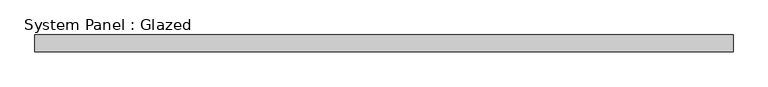
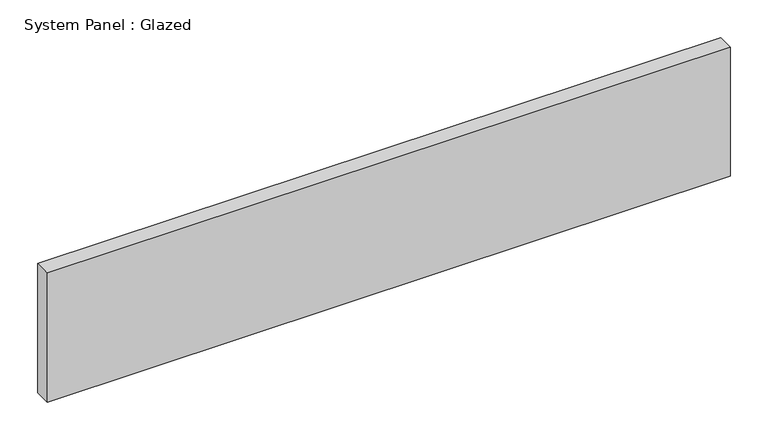
"""IFC4 building model written with IfcOpenShell, lengths in millimetres: plate geometry, System Panel : Glazed."""

from ifc_helpers import new_model, si_unit, origin, origin_with_axes, place, context, project, spatial, polyline, outline, extrude, source, transform, mapped, element, save


def system_panel_glazed_6ba3ac31(model_context):
    return source(origin(), model_context, "Body", "SweptSolid", [
        extrude(outline(polyline([(523.875, 19.05), (-523.875, 19.05), (-523.875, 44.45), (523.875, 44.45), (523.875, 19.05)])), origin_with_axes(), (0.0, 0.0, 1.0), 209.55),
    ])


if __name__ == "__main__":
    model = new_model("IFC4")
    model_context = context("Model", 3, world=origin())
    ifc_project = project(units=[si_unit("LENGTHUNIT", "METRE", prefix="MILLI")], contexts=[model_context])
    site = spatial("IfcSite", under=ifc_project)
    building = spatial("IfcBuilding", under=site)
    placement = place(None, origin())
    system_panel_glazed_shape = system_panel_glazed_6ba3ac31(model_context)
    element("IfcPlate", 1, ObjectType="System Panel : Glazed", at=placement, inside=building, context=model_context, shape_type="MappedRepresentation", body=[
        mapped(system_panel_glazed_shape, transform((0.0, 0.0, 0.0), x_axis=(1.0, 0.0, 0.0), y_axis=(0.0, 1.0, 0.0), z_axis=(0.0, 0.0, 1.0))),
    ])
    save(model, "model.ifc")

# Revit data of these elements
# Type "System Panel : Glazed"
#   Construction Type Id = "GSP4R"
#   Analytic Construction = "1/8 in Pilkington single glazing"
#   Visual Light Transmittance = 0.9
#   Solar Heat Gain Coefficient = 0.86
#   Heat Transfer Coefficient (U) = 1.18115 BTU/(h·ft²·°F)
#   Define Thermal Properties by = 1
# Element 1 (IfcPlate, "System Panel : Glazed")
#   Materials on its faces: "Glass"
# Materials
#   "Glass": class "Glass", colour RGB 0 128 192, transparency 0.75, Description = "Soda Lime Glass", Cost = 0
